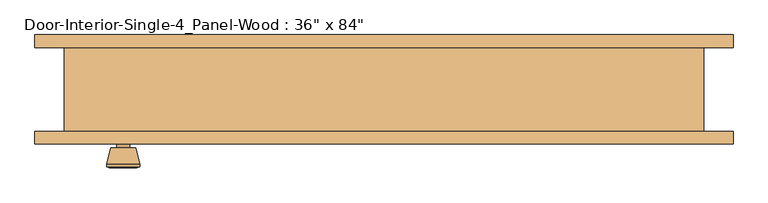
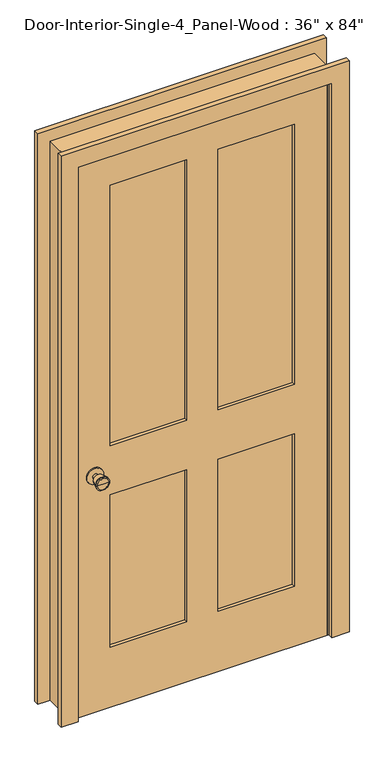
"""IFC4 building model written with IfcOpenShell, lengths in millimetres: door geometry."""

from ifc_helpers import new_model, si_unit, point, frame, frame_2d, origin, place, context, project, spatial, polyline, circle_curve, trimmed, segment, composite_curve, outline, extrude, faceted_brep, source, transform, mapped, element, save
from ifc_brep_helpers import plane_surface, cylinder_surface, revolved_surface, advanced_brep


def door_a823658d(model_context):
    return source(origin(), model_context, "Body", "SolidModel", [
        advanced_brep(
        [(-393.7, -19.4, 914.4), (-403.7, -19.4, 914.4), (-383.7, -19.4, 914.4), (-373.2241324, 29.6, 914.4), (-414.1758676, 29.6, 914.4), (-393.7, 29.6, 914.4), (-368.7, 27.7721319, 914.4), (-418.7, 27.7721319, 914.4), (-368.7, 24.3084537, 914.4), (-418.7, 24.3084537, 914.4), (-375.063764, -0.4, 914.4), (-412.336236, -0.4, 914.4), (-383.7, -0.4, 914.4), (-403.7, -0.4, 914.4)],
        [
            (0, 1),
            (1, 2, circle_curve(frame((-393.7, -19.4, 914.4), z_axis=(0.0, -1.0, 0.0), x_axis=(-1.0, 0.0, 0.0)), 10.0)),
            (2, 0),
            (2, 1, circle_curve(frame((-393.7, -19.4, 914.4), z_axis=(0.0, -1.0, 0.0), x_axis=(-1.0, 0.0, 0.0)), 10.0)),
            (3, 4, circle_curve(frame((-393.7, 29.6, 914.4), z_axis=(0.0, 1.0, 0.0), x_axis=(-1.0, 0.0, 0.0)), 20.4758676)),
            (4, 5),
            (5, 3),
            (4, 3, circle_curve(frame((-393.7, 29.6, 914.4), z_axis=(0.0, 1.0, 0.0), x_axis=(-1.0, 0.0, 0.0)), 20.4758676)),
            (6, 7, circle_curve(frame((-393.7, 27.7721319, 914.4), z_axis=(0.0, 1.0, 0.0), x_axis=(-1.0, 0.0, 0.0)), 25.0)),
            (7, 4),
            (3, 6),
            (7, 6, circle_curve(frame((-393.7, 27.7721319, 914.4), z_axis=(0.0, 1.0, 0.0), x_axis=(-1.0, 0.0, 0.0)), 25.0)),
            (8, 9, circle_curve(frame((-393.7, 24.3084537, 914.4), z_axis=(0.0, 1.0, 0.0), x_axis=(-1.0, 0.0, 0.0)), 25.0)),
            (9, 7),
            (6, 8),
            (9, 8, circle_curve(frame((-393.7, 24.3084537, 914.4), z_axis=(0.0, 1.0, 0.0), x_axis=(-1.0, 0.0, 0.0)), 25.0)),
            (10, 11, circle_curve(frame((-393.7, -0.4, 914.4), z_axis=(0.0, 1.0, 0.0), x_axis=(-1.0, 0.0, 0.0)), 18.636236)),
            (11, 9),
            (8, 10),
            (11, 10, circle_curve(frame((-393.7, -0.4, 914.4), z_axis=(0.0, 1.0, 0.0), x_axis=(-1.0, 0.0, 0.0)), 18.636236)),
            (12, 13, circle_curve(frame((-393.7, -0.4, 914.4), z_axis=(0.0, 1.0, 0.0), x_axis=(-1.0, 0.0, 0.0)), 10.0)),
            (13, 11),
            (10, 12),
            (13, 12, circle_curve(frame((-393.7, -0.4, 914.4), z_axis=(0.0, 1.0, 0.0), x_axis=(-1.0, 0.0, 0.0)), 10.0)),
            (1, 13),
            (12, 2),
        ],
        [
            plane_surface(frame((-393.7, -19.4, 914.4), z_axis=(0.0, -1.0, 0.0), x_axis=(-1.0, 0.0, 0.0))),
            plane_surface(frame((-393.7, 29.6, 914.4), z_axis=(0.0, 1.0, 0.0), x_axis=(-1.0, 0.0, 0.0))),
            revolved_surface(polyline([(-414.1758676, 29.6, 914.4), (-418.7, 27.7721319, 914.4)]), (-393.7, -19.4, 914.4), (0.0, -1.0, 0.0)),
            cylinder_surface(frame((-393.7, -19.4, 914.4), z_axis=(0.0, -1.0, 0.0), x_axis=(-1.0, 0.0, 0.0)), 25.0),
            revolved_surface(polyline([(-418.7, 24.3084537, 914.4), (-412.336236, -0.4, 914.4)]), (-393.7, -19.4, 914.4), (0.0, -1.0, 0.0)),
            plane_surface(frame((-393.7, -0.4, 914.4), z_axis=(0.0, -1.0, 0.0), x_axis=(-1.0, 0.0, 0.0))),
            cylinder_surface(frame((-393.7, -19.4, 914.4), z_axis=(0.0, -1.0, 0.0), x_axis=(-1.0, 0.0, 0.0)), 10.0),
        ],
        [
            (0, [[1, 2, 3]]),
            (0, [[-3, 4, -1]]),
            (1, [[5, 6, 7]]),
            (1, [[8, -7, -6]]),
            (2, [[9, 10, -5, 11]]),
            (2, [[12, -11, -8, -10]]),
            (3, [[13, 14, -9, 15]]),
            (3, [[16, -15, -12, -14]]),
            (4, [[17, 18, -13, 19]]),
            (4, [[20, -19, -16, -18]]),
            (5, [[21, 22, -17, 23]]),
            (5, [[24, -23, -20, -22]]),
            (6, [[-2, 25, -21, 26]]),
            (6, [[-4, -26, -24, -25]]),
        ],
    ),
        extrude(outline(composite_curve([segment(trimmed(circle_curve(frame_2d((914.4, -393.7)), 30.0), [point((914.4, -423.7))], [point((914.4, -363.7))], False, "CARTESIAN"), True, "CONTINUOUS"), segment(trimmed(circle_curve(frame_2d((914.4, -393.7)), 30.0), [point((914.4, -363.7))], [point((914.4, -423.7))], False, "CARTESIAN"), True, "CONTINUOUS")], self_intersect=False)), frame((0.0, -25.4, 0.0), z_axis=(0.0, 1.0, 0.0), x_axis=(0.0, 0.0, 1.0)), (0.0, 0.0, 1.0), 6.0),
        advanced_brep(
        [(-393.7, -66.325, 914.4), (-383.7, -66.325, 914.4), (-403.7, -66.325, 914.4), (-373.2241324, -115.325, 914.4), (-393.7, -115.325, 914.4), (-414.1758676, -115.325, 914.4), (-368.7, -113.4971319, 914.4), (-418.7, -113.4971319, 914.4), (-368.7, -110.0334537, 914.4), (-418.7, -110.0334537, 914.4), (-375.063764, -85.325, 914.4), (-412.336236, -85.325, 914.4), (-383.7, -85.325, 914.4), (-403.7, -85.325, 914.4)],
        [
            (0, 1),
            (1, 2, circle_curve(frame((-393.7, -66.325, 914.4), z_axis=(0.0, 1.0, 0.0), x_axis=(-1.0, 0.0, 0.0)), 10.0)),
            (2, 0),
            (2, 1, circle_curve(frame((-393.7, -66.325, 914.4), z_axis=(0.0, 1.0, 0.0), x_axis=(-1.0, 0.0, 0.0)), 10.0)),
            (3, 4),
            (4, 5),
            (5, 3, circle_curve(frame((-393.7, -115.325, 914.4), z_axis=(0.0, -1.0, 0.0), x_axis=(-1.0, 0.0, 0.0)), 20.4758676)),
            (3, 5, circle_curve(frame((-393.7, -115.325, 914.4), z_axis=(0.0, -1.0, 0.0), x_axis=(-1.0, 0.0, 0.0)), 20.4758676)),
            (6, 3),
            (5, 7),
            (7, 6, circle_curve(frame((-393.7, -113.4971319, 914.4), z_axis=(0.0, -1.0, 0.0), x_axis=(-1.0, 0.0, 0.0)), 25.0)),
            (6, 7, circle_curve(frame((-393.7, -113.4971319, 914.4), z_axis=(0.0, -1.0, 0.0), x_axis=(-1.0, 0.0, 0.0)), 25.0)),
            (8, 6),
            (7, 9),
            (9, 8, circle_curve(frame((-393.7, -110.0334537, 914.4), z_axis=(0.0, -1.0, 0.0), x_axis=(-1.0, 0.0, 0.0)), 25.0)),
            (8, 9, circle_curve(frame((-393.7, -110.0334537, 914.4), z_axis=(0.0, -1.0, 0.0), x_axis=(-1.0, 0.0, 0.0)), 25.0)),
            (10, 8),
            (9, 11),
            (11, 10, circle_curve(frame((-393.7, -85.325, 914.4), z_axis=(0.0, -1.0, 0.0), x_axis=(-1.0, 0.0, 0.0)), 18.636236)),
            (10, 11, circle_curve(frame((-393.7, -85.325, 914.4), z_axis=(0.0, -1.0, 0.0), x_axis=(-1.0, 0.0, 0.0)), 18.636236)),
            (12, 10),
            (11, 13),
            (13, 12, circle_curve(frame((-393.7, -85.325, 914.4), z_axis=(0.0, -1.0, 0.0), x_axis=(-1.0, 0.0, 0.0)), 10.0)),
            (12, 13, circle_curve(frame((-393.7, -85.325, 914.4), z_axis=(0.0, -1.0, 0.0), x_axis=(-1.0, 0.0, 0.0)), 10.0)),
            (1, 12),
            (13, 2),
        ],
        [
            plane_surface(frame((-393.7, -66.325, 914.4), z_axis=(0.0, 1.0, 0.0), x_axis=(-1.0, 0.0, 0.0))),
            plane_surface(frame((-393.7, -115.325, 914.4), z_axis=(0.0, -1.0, 0.0), x_axis=(-1.0, 0.0, 0.0))),
            revolved_surface(polyline([(-414.1758676, -115.325, 914.4), (-418.7, -113.4971319, 914.4)]), (-393.7, -66.325, 914.4), (0.0, 1.0, 0.0)),
            cylinder_surface(frame((-393.7, -66.325, 914.4), z_axis=(0.0, 1.0, 0.0), x_axis=(-1.0, 0.0, 0.0)), 25.0),
            revolved_surface(polyline([(-418.7, -110.0334537, 914.4), (-412.336236, -85.325, 914.4)]), (-393.7, -66.325, 914.4), (0.0, 1.0, 0.0)),
            plane_surface(frame((-393.7, -85.325, 914.4), z_axis=(0.0, 1.0, 0.0), x_axis=(-1.0, 0.0, 0.0))),
            cylinder_surface(frame((-393.7, -66.325, 914.4), z_axis=(0.0, 1.0, 0.0), x_axis=(-1.0, 0.0, 0.0)), 10.0),
        ],
        [
            (0, [[1, 2, 3]]),
            (0, [[-3, 4, -1]]),
            (1, [[5, 6, 7]]),
            (1, [[-6, -5, 8]]),
            (2, [[9, -7, 10, 11]]),
            (2, [[-10, -8, -9, 12]]),
            (3, [[13, -11, 14, 15]]),
            (3, [[-14, -12, -13, 16]]),
            (4, [[17, -15, 18, 19]]),
            (4, [[-18, -16, -17, 20]]),
            (5, [[21, -19, 22, 23]]),
            (5, [[-22, -20, -21, 24]]),
            (6, [[25, -23, 26, -2]]),
            (6, [[-26, -24, -25, -4]]),
        ],
    ),
        extrude(outline(composite_curve([segment(trimmed(circle_curve(frame_2d((914.4, -393.7)), 30.0), [point((914.4, -423.7))], [point((914.4, -363.7))], False, "CARTESIAN"), True, "CONTINUOUS"), segment(trimmed(circle_curve(frame_2d((914.4, -393.7)), 30.0), [point((914.4, -363.7))], [point((914.4, -423.7))], False, "CARTESIAN"), True, "CONTINUOUS")], self_intersect=False)), frame((0.0, -66.325, 0.0), z_axis=(0.0, 1.0, 0.0), x_axis=(0.0, 0.0, 1.0)), (0.0, 0.0, 1.0), 6.0),
        faceted_brep([(482.6, -60.325, 0.0), (457.2, -60.325, 0.0), (457.2, -25.4, 0.0), (444.5, -25.4, 0.0), (444.5, 9.525, 0.0), (457.2, 9.525, 0.0), (457.2, 66.675, 0.0), (482.6, 66.675, 0.0), (482.6, 66.675, 2159.0), (482.6, -60.325, 2159.0), (457.2, 66.675, 2133.6), (-457.2, 66.675, 2133.6), (-457.2, 66.675, 0.0), (-482.6, 66.675, 0.0), (-482.6, 66.675, 2159.0), (457.2, 9.525, 2133.6), (444.5, 9.525, 2120.9), (-444.5, 9.525, 2120.9), (-444.5, 9.525, 0.0), (-457.2, 9.525, 0.0), (-457.2, 9.525, 2133.6), (444.5, -25.4, 2120.9), (457.2, -25.4, 2133.6), (-457.2, -25.4, 2133.6), (-457.2, -25.4, 0.0), (-444.5, -25.4, 0.0), (-444.5, -25.4, 2120.9), (457.2, -60.325, 2133.6), (-482.6, -60.325, 2159.0), (-482.6, -60.325, 0.0), (-457.2, -60.325, 0.0), (-457.2, -60.325, 2133.6)], [[[0, 1, 2, 3, 4, 5, 6, 7]], [[7, 8, 9, 0]], [[6, 10, 11, 12, 13, 14, 8, 7]], [[5, 15, 10, 6]], [[4, 16, 17, 18, 19, 20, 15, 5]], [[3, 21, 16, 4]], [[2, 22, 23, 24, 25, 26, 21, 3]], [[1, 27, 22, 2]], [[0, 9, 28, 29, 30, 31, 27, 1]], [[8, 14, 28, 9]], [[15, 20, 11, 10]], [[21, 26, 17, 16]], [[27, 31, 23, 22]], [[29, 13, 12, 19, 18, 25, 24, 30]], [[14, 13, 29, 28]], [[20, 19, 12, 11]], [[26, 25, 18, 17]], [[31, 30, 24, 23]]]),
        extrude(outline(polyline([(2133.6, -457.2), (0.0, -457.2), (0.0, 457.2), (2133.6, 457.2), (2133.6, -457.2)]), holes=[polyline([(2014.5375, 57.15), (2014.5375, 336.55), (1009.65, 336.55), (1009.65, 57.15), (2014.5375, 57.15)]), polyline([(1009.65, -57.15), (1009.65, -336.55), (2014.5375, -336.55), (2014.5375, -57.15), (1009.65, -57.15)]), polyline([(819.15, 57.15), (819.15, 336.55), (231.775, 336.55), (231.775, 57.15), (819.15, 57.15)]), polyline([(231.775, -57.15), (231.775, -336.55), (819.15, -336.55), (819.15, -57.15), (231.775, -57.15)])]), frame((0.0, -60.325, 0.0), z_axis=(0.0, 1.0, 0.0), x_axis=(0.0, 0.0, 1.0)), (0.0, 0.0, 1.0), 34.925),
        extrude(outline(polyline([(336.55, -37.0416667), (336.55, -48.6833333), (57.15, -48.6833333), (57.15, -37.0416667), (336.55, -37.0416667)])), frame((0.0, 0.0, 1009.65), z_axis=(0.0, 0.0, 1.0), x_axis=(1.0, 0.0, 0.0)), (0.0, 0.0, 1.0), 1004.8875),
        extrude(outline(polyline([(-57.15, -37.0416667), (-57.15, -48.6833333), (-336.55, -48.6833333), (-336.55, -37.0416667), (-57.15, -37.0416667)])), frame((0.0, 0.0, 1009.65), z_axis=(0.0, 0.0, 1.0), x_axis=(1.0, 0.0, 0.0)), (0.0, 0.0, 1.0), 1004.8875),
        extrude(outline(polyline([(336.55, -37.0416667), (336.55, -48.6833333), (57.15, -48.6833333), (57.15, -37.0416667), (336.55, -37.0416667)])), frame((0.0, 0.0, 231.775), z_axis=(0.0, 0.0, 1.0), x_axis=(1.0, 0.0, 0.0)), (0.0, 0.0, 1.0), 587.375),
        extrude(outline(polyline([(-57.15, -37.0416667), (-57.15, -48.6833333), (-336.55, -48.6833333), (-336.55, -37.0416667), (-57.15, -37.0416667)])), frame((0.0, 0.0, 231.775), z_axis=(0.0, 0.0, 1.0), x_axis=(1.0, 0.0, 0.0)), (0.0, 0.0, 1.0), 587.375),
        extrude(outline(polyline([(0.0, 527.05), (2203.45, 527.05), (2203.45, -527.05), (0.0, -527.05), (0.0, -463.55), (2139.95, -463.55), (2139.95, 463.55), (0.0, 463.55), (0.0, 527.05)])), frame((0.0, -79.375, 0.0), z_axis=(0.0, 1.0, 0.0), x_axis=(0.0, 0.0, 1.0)), (0.0, 0.0, 1.0), 19.05),
        extrude(outline(polyline([(0.0, 527.05), (2203.45, 527.05), (2203.45, -527.05), (0.0, -527.05), (0.0, -463.55), (2139.95, -463.55), (2139.95, 463.55), (0.0, 463.55), (0.0, 527.05)])), frame((0.0, 66.675, 0.0), z_axis=(0.0, 1.0, 0.0), x_axis=(0.0, 0.0, 1.0)), (0.0, 0.0, 1.0), 19.05),
    ])


if __name__ == "__main__":
    model = new_model("IFC4")
    model_context = context("Model", 3, world=origin())
    ifc_project = project(units=[si_unit("LENGTHUNIT", "METRE", prefix="MILLI")], contexts=[model_context])
    site = spatial("IfcSite", under=ifc_project)
    building = spatial("IfcBuilding", under=site)
    placement = place(None, origin())
    door_shape = door_a823658d(model_context)
    element("IfcDoor", 1, ObjectType="Door-Interior-Single-4_Panel-Wood : 36\" x 84\"", at=placement, inside=building, context=model_context, shape_type="MappedRepresentation", body=[
        mapped(door_shape, transform((0.0, 0.0, 0.0), x_axis=(1.0, 0.0, 0.0), y_axis=(0.0, 1.0, 0.0), z_axis=(0.0, 0.0, 1.0))),
    ])
    save(model, "model.ifc")

# Revit data of these elements
# Type "Door-Interior-Single-4_Panel-Wood : 36\" x 84\""
#   Type Mark = "9"
#   Assembly Code = "C1020300"
#   Analytic Construction = "Wooden"
#   Top Rail = 0' - 4 11/16"
#   Thickness = 0' - 1 3/8"
#   Thermal Resistance (R) = 2.5876 (h·ft²·°F)/BTU
#   Swing Angle [instance default] = 90.00°
#   Stiles = 0' - 4 3/4"
#   Rough Width = 3' - 2"
#   Rough Height = 7' - 1"
#   Mullion = 0' - 4 1/2"
#   Lock Rail = 0' - 7 1/2"
#   Height = 7' - 0"
#   Width = 3' - 0"
#   Heat Transfer Coefficient (U) = 0.3865 BTU/(h·ft²·°F)
#   Bottom Rail = 0' - 9 1/8"
#   Trim Material = Cherry
#   Panel Material = Cherry
#   Frame Material = Cherry
#   Door Handle Material = Aluminum
#   Visual Light Transmittance = 0
#   Solar Heat Gain Coefficient = 0
#   Wall Closure = (empty or 0)
#   Function = (empty or 0)
# Element 1 (IfcDoor, "Door-Interior-Single-4_Panel-Wood : 36\" x 84\"")
#   Materials on its faces: "Cherry", "Aluminum"
# Materials
#   "Cherry": class "Wood", colour RGB 226 177 128, transparency 0, Description = "Prunus Serotina", Cost = 0
#   "Aluminum": class "Metal", colour RGB 247 247 247, transparency 0, Description = "Aluminum 6061", Cost = 0
